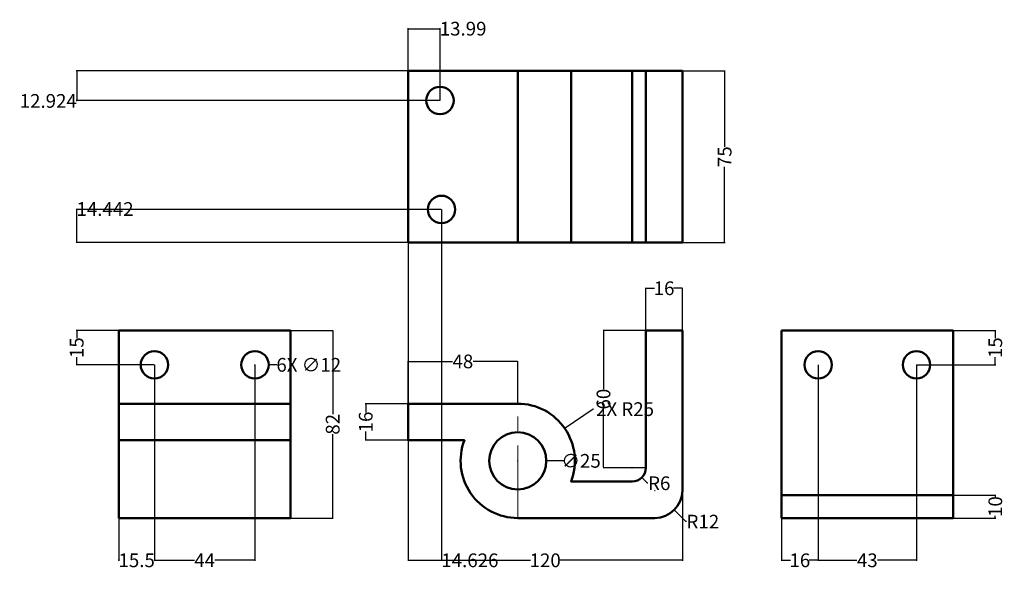
# Model space of a CAD drawing. Units: millimetres. Extents: x -15 to 416, y 9 to 249.
import ezdxf

# ---------------------------------------------------------------- set-up
doc = ezdxf.new("R2010")
doc.units = ezdxf.units.MM
doc.header["$MEASUREMENT"] = 0
doc.linetypes.add('CENTER', pattern=[50.8, 31.75, -6.35, 6.35, -6.35])
for name, color, linetype, lineweight in [('M-CNTR', 1, 'CENTER', 18), ('M-DIMS', 2, 'Continuous', 18), ('M-OUTL', 7, 'Continuous', 50)]:
    doc.layers.add(name, color=color, linetype=linetype, lineweight=lineweight)
doc.styles.get("Standard").update_dxf_attribs({"font": 'arial.ttf'})
doc.dimstyles.get("Standard").update_dxf_attribs({"dimtxt": 6, "dimasz": 0.18, "dimexe": 0.18, "dimexo": 0.0625, "dimgap": 0.09, "dimtad": 0, "dimtoh": 1, "dimdec": 0, "dimzin": 0, "dimdsep": 46, "dimtxsty": 'Standard', "dimcen": 0.09, "dimadec": 0, "dimazin": 0, "dimtfac": 1, "dimtdec": 0, "dimtofl": 0, "dimtmove": 0, "dimatfit": 3, "dimfxl": 1, "dimtolj": 1, "dimtzin": 0, "dimarcsym": 0})

# ---------------------------------------------------------------- blocks, each defined once
blk = doc.blocks.new('MTG-HOLE-D12')
blk.add_circle((6, 6), 6)
blk = doc.blocks.new('*D2')
at = {"layer": 'Defpoints', "color": 0, "transparency": 16777216}
for p in [(154.95, 65.07), (274.95, 43.07), (274.95, 12.57)]:
    blk.add_point(p, dxfattribs=at)
at = {"layer": 'M-DIMS', "color": 0, "lineweight": -2, "transparency": 16777216}
for p, q in [((154.95, 65.01), (154.95, 12.39)), ((274.95, 43.01), (274.95, 12.39)), ((155.13, 12.57), (208.52, 12.57)), ((274.77, 12.57), (221.37, 12.57))]:
    blk.add_line(p, q, dxfattribs=at)
at = {"layer": 'M-DIMS', "color": 0, "transparency": 16777216}
for points in [[(155.13, 12.6), (155.13, 12.54), (154.95, 12.57)], [(274.77, 12.6), (274.77, 12.54), (274.95, 12.57)]]:
    blk.add_solid(points, dxfattribs=at)
at = {"layer": 'M-DIMS', "color": 0, "transparency": 16777216, "insert": (214.95, 12.57), "char_height": 6, "attachment_point": 5}
blk.add_mtext('\\A1;120', dxfattribs=at)
blk = doc.blocks.new('*D3')
at = {"layer": 'Defpoints', "color": 0, "transparency": 16777216}
for p in [(103.5, 113.07), (103.5, 31.07), (122, 31.07)]:
    blk.add_point(p, dxfattribs=at)
at = {"layer": 'M-DIMS', "color": 0, "lineweight": -2, "transparency": 16777216}
for p, q in [((103.56, 113.07), (122.18, 113.07)), ((122, 112.89), (122, 76.43)), ((122, 31.25), (122, 67.71)), ((103.56, 31.07), (122.18, 31.07))]:
    blk.add_line(p, q, dxfattribs=at)
at = {"layer": 'M-DIMS', "color": 0, "transparency": 16777216}
for points in [[(121.97, 112.89), (122.03, 112.89), (122, 113.07)], [(121.97, 31.25), (122.03, 31.25), (122, 31.07)]]:
    blk.add_solid(points, dxfattribs=at)
at = {"layer": 'M-DIMS', "color": 0, "transparency": 16777216, "insert": (122, 72.07), "char_height": 6, "attachment_point": 5, "rotation": 90}
blk.add_mtext('\\A1;82', dxfattribs=at)
blk = doc.blocks.new('*D4')
at = {"layer": 'Defpoints', "color": 0, "transparency": 16777216}
for p in [(274.95, 226.61), (274.95, 151.61), (293.45, 151.61)]:
    blk.add_point(p, dxfattribs=at)
at = {"layer": 'M-DIMS', "color": 0, "lineweight": -2, "transparency": 16777216}
for p, q in [((275.01, 226.61), (293.63, 226.61)), ((293.45, 226.43), (293.45, 193.49)), ((293.45, 151.79), (293.45, 184.72)), ((275.01, 151.61), (293.63, 151.61))]:
    blk.add_line(p, q, dxfattribs=at)
at = {"layer": 'M-DIMS', "color": 0, "transparency": 16777216}
for points in [[(293.42, 226.43), (293.48, 226.43), (293.45, 226.61)], [(293.42, 151.79), (293.48, 151.79), (293.45, 151.61)]]:
    blk.add_solid(points, dxfattribs=at)
at = {"layer": 'M-DIMS', "color": 0, "transparency": 16777216, "insert": (293.45, 189.11), "char_height": 6, "attachment_point": 5, "rotation": 90}
blk.add_mtext('\\A1;75', dxfattribs=at)
blk = doc.blocks.new('*D5')
at = {"layer": 'Defpoints', "color": 0, "transparency": 16777216}
for p in [(202.95, 99.57), (154.95, 81.07), (202.95, 81.07)]:
    blk.add_point(p, dxfattribs=at)
at = {"layer": 'M-DIMS', "color": 0, "lineweight": -2, "transparency": 16777216}
for p, q in [((154.95, 81.13), (154.95, 99.75)), ((155.13, 99.57), (174.43, 99.57)), ((202.77, 99.57), (183.46, 99.57)), ((202.95, 81.13), (202.95, 99.75))]:
    blk.add_line(p, q, dxfattribs=at)
at = {"layer": 'M-DIMS', "color": 0, "transparency": 16777216}
for points in [[(155.13, 99.6), (155.13, 99.54), (154.95, 99.57)], [(202.77, 99.6), (202.77, 99.54), (202.95, 99.57)]]:
    blk.add_solid(points, dxfattribs=at)
at = {"layer": 'M-DIMS', "color": 0, "transparency": 16777216, "insert": (178.95, 99.57), "char_height": 6, "attachment_point": 5}
blk.add_mtext('\\A1;48', dxfattribs=at)
blk = doc.blocks.new('*D6')
at = {"layer": 'Defpoints', "color": 0, "transparency": 16777216}
for p in [(136.45, 81.07), (154.95, 81.07), (154.95, 65.07)]:
    blk.add_point(p, dxfattribs=at)
at = {"layer": 'M-DIMS', "color": 0, "lineweight": -2, "transparency": 16777216}
for p, q in [((154.88, 81.07), (136.27, 81.07)), ((136.45, 80.89), (136.45, 77.17)), ((136.45, 65.25), (136.45, 68.97)), ((154.88, 65.07), (136.27, 65.07))]:
    blk.add_line(p, q, dxfattribs=at)
at = {"layer": 'M-DIMS', "color": 0, "transparency": 16777216}
for points in [[(136.42, 80.89), (136.48, 80.89), (136.45, 81.07)], [(136.42, 65.25), (136.48, 65.25), (136.45, 65.07)]]:
    blk.add_solid(points, dxfattribs=at)
at = {"layer": 'M-DIMS', "color": 0, "transparency": 16777216, "insert": (136.45, 73.07), "char_height": 6, "attachment_point": 5, "rotation": 90}
blk.add_mtext('\\A1;16', dxfattribs=at)
blk = doc.blocks.new('*D7')
at = {"layer": 'Defpoints', "color": 0, "transparency": 16777216}
for p in [(274.95, 131.57), (258.95, 113.07), (274.95, 113.07)]:
    blk.add_point(p, dxfattribs=at)
at = {"layer": 'M-DIMS', "color": 0, "lineweight": -2, "transparency": 16777216}
for p, q in [((258.95, 113.13), (258.95, 131.75)), ((259.13, 131.57), (262.84, 131.57)), ((274.77, 131.57), (271.05, 131.57)), ((274.95, 113.13), (274.95, 131.75))]:
    blk.add_line(p, q, dxfattribs=at)
at = {"layer": 'M-DIMS', "color": 0, "transparency": 16777216}
for points in [[(259.13, 131.6), (259.13, 131.54), (258.95, 131.57)], [(274.77, 131.6), (274.77, 131.54), (274.95, 131.57)]]:
    blk.add_solid(points, dxfattribs=at)
at = {"layer": 'M-DIMS', "color": 0, "transparency": 16777216, "insert": (266.95, 131.57), "char_height": 6, "attachment_point": 5}
blk.add_mtext('\\A1;16', dxfattribs=at)
blk = doc.blocks.new('*D8')
at = {"layer": 'Defpoints', "color": 0, "transparency": 16777216}
for p in [(240.45, 113.07), (258.95, 113.07), (258.95, 53.07)]:
    blk.add_point(p, dxfattribs=at)
at = {"layer": 'M-DIMS', "color": 0, "lineweight": -2, "transparency": 16777216}
for p, q in [((258.88, 113.07), (240.27, 113.07)), ((240.45, 112.89), (240.45, 87.46)), ((240.45, 53.25), (240.45, 78.68)), ((258.88, 53.07), (240.27, 53.07))]:
    blk.add_line(p, q, dxfattribs=at)
at = {"layer": 'M-DIMS', "color": 0, "transparency": 16777216}
for points in [[(240.42, 112.89), (240.48, 112.89), (240.45, 113.07)], [(240.42, 53.25), (240.48, 53.25), (240.45, 53.07)]]:
    blk.add_solid(points, dxfattribs=at)
at = {"layer": 'M-DIMS', "color": 0, "transparency": 16777216, "insert": (240.45, 83.07), "char_height": 6, "attachment_point": 5, "rotation": 90}
blk.add_mtext('\\A1;60', dxfattribs=at)
blk = doc.blocks.new('*D9')
at = {"layer": 'Defpoints', "color": 0, "transparency": 16777216}
for p in [(43.999556, 98.070817), (28.499556, 31.070817), (43.999556, 12.570817)]:
    blk.add_point(p, dxfattribs=at)
at = {"layer": 'M-DIMS', "color": 0, "lineweight": -2, "transparency": 16777216}
for p, q in [((43.999556, 98.008317), (43.999556, 12.390817)), ((28.499556, 31.008317), (28.499556, 12.390817)), ((28.319556, 12.570817), (28.139556, 12.570817)), ((44.179556, 12.570817), (44.359556, 12.570817))]:
    blk.add_line(p, q, dxfattribs=at)
at = {"layer": 'M-DIMS', "color": 0, "transparency": 16777216}
for points in [[(28.319556, 12.600817), (28.319556, 12.540817), (28.499556, 12.570817)], [(44.179556, 12.600817), (44.179556, 12.540817), (43.999556, 12.570817)]]:
    blk.add_solid(points, dxfattribs=at)
at = {"layer": 'M-DIMS', "color": 0, "transparency": 16777216, "insert": (36.249556, 12.570817), "char_height": 6, "attachment_point": 5}
blk.add_mtext('\\A1;15.5', dxfattribs=at)
blk = doc.blocks.new('*D10')
at = {"layer": 'Defpoints', "color": 0, "transparency": 16777216}
for p in [(44, 98.07), (88, 98.07), (88, 12.57)]:
    blk.add_point(p, dxfattribs=at)
at = {"layer": 'M-DIMS', "color": 0, "lineweight": -2, "transparency": 16777216}
for p, q in [((44, 98.01), (44, 12.39)), ((88, 98.01), (88, 12.39)), ((44.18, 12.57), (61.5, 12.57)), ((87.82, 12.57), (70.5, 12.57))]:
    blk.add_line(p, q, dxfattribs=at)
at = {"layer": 'M-DIMS', "color": 0, "transparency": 16777216}
for points in [[(44.18, 12.6), (44.18, 12.54), (44, 12.57)], [(87.82, 12.6), (87.82, 12.54), (88, 12.57)]]:
    blk.add_solid(points, dxfattribs=at)
at = {"layer": 'M-DIMS', "color": 0, "transparency": 16777216, "insert": (66, 12.57), "char_height": 6, "attachment_point": 5}
blk.add_mtext('\\A1;44', dxfattribs=at)
blk = doc.blocks.new('*D11')
at = {"layer": 'Defpoints', "color": 0, "transparency": 16777216}
for p in [(28.5, 113.07), (10, 98.07), (44, 98.07)]:
    blk.add_point(p, dxfattribs=at)
at = {"layer": 'M-DIMS', "color": 0, "lineweight": -2, "transparency": 16777216}
for p, q in [((28.44, 113.07), (9.82, 113.07)), ((10, 112.89), (10, 109.7)), ((10, 98.25), (10, 101.44)), ((43.94, 98.07), (9.82, 98.07))]:
    blk.add_line(p, q, dxfattribs=at)
at = {"layer": 'M-DIMS', "color": 0, "transparency": 16777216}
for points in [[(9.97, 112.89), (10.03, 112.89), (10, 113.07)], [(9.97, 98.25), (10.03, 98.25), (10, 98.07)]]:
    blk.add_solid(points, dxfattribs=at)
at = {"layer": 'M-DIMS', "color": 0, "transparency": 16777216, "insert": (10, 105.57), "char_height": 6, "attachment_point": 5, "rotation": 90}
blk.add_mtext('\\A1;15', dxfattribs=at)
blk = doc.blocks.new('*D12')
at = {"layer": 'Defpoints', "color": 0, "transparency": 16777216}
for p in [(334.35, 98.07), (318.35, 31.07), (334.35, 12.57)]:
    blk.add_point(p, dxfattribs=at)
at = {"layer": 'M-DIMS', "color": 0, "lineweight": -2, "transparency": 16777216}
for p, q in [((334.35, 98.01), (334.35, 12.39)), ((318.35, 31.01), (318.35, 12.39)), ((318.53, 12.57), (322.25, 12.57)), ((334.17, 12.57), (330.45, 12.57))]:
    blk.add_line(p, q, dxfattribs=at)
at = {"layer": 'M-DIMS', "color": 0, "transparency": 16777216}
for points in [[(318.53, 12.6), (318.53, 12.54), (318.35, 12.57)], [(334.17, 12.6), (334.17, 12.54), (334.35, 12.57)]]:
    blk.add_solid(points, dxfattribs=at)
at = {"layer": 'M-DIMS', "color": 0, "transparency": 16777216, "insert": (326.35, 12.57), "char_height": 6, "attachment_point": 5}
blk.add_mtext('\\A1;16', dxfattribs=at)
blk = doc.blocks.new('*D13')
at = {"layer": 'Defpoints', "color": 0, "transparency": 16777216}
for p in [(334.35, 98.07), (377.35, 98.07), (377.35, 12.57)]:
    blk.add_point(p, dxfattribs=at)
at = {"layer": 'M-DIMS', "color": 0, "lineweight": -2, "transparency": 16777216}
for p, q in [((334.35, 98.01), (334.35, 12.39)), ((377.35, 98.01), (377.35, 12.39)), ((334.53, 12.57), (351.34, 12.57)), ((377.17, 12.57), (360.36, 12.57))]:
    blk.add_line(p, q, dxfattribs=at)
at = {"layer": 'M-DIMS', "color": 0, "transparency": 16777216}
for points in [[(334.53, 12.6), (334.53, 12.54), (334.35, 12.57)], [(377.17, 12.6), (377.17, 12.54), (377.35, 12.57)]]:
    blk.add_solid(points, dxfattribs=at)
at = {"layer": 'M-DIMS', "color": 0, "transparency": 16777216, "insert": (355.85, 12.57), "char_height": 6, "attachment_point": 5}
blk.add_mtext('\\A1;43', dxfattribs=at)
blk = doc.blocks.new('*D14')
at = {"layer": 'Defpoints', "color": 0, "transparency": 16777216}
for p in [(393.35, 113.07), (411.85, 113.07), (377.35, 98.07)]:
    blk.add_point(p, dxfattribs=at)
at = {"layer": 'M-DIMS', "color": 0, "lineweight": -2, "transparency": 16777216}
for p, q in [((393.41, 113.07), (412.03, 113.07)), ((411.85, 112.89), (411.85, 109.7)), ((411.85, 98.25), (411.85, 101.44)), ((377.41, 98.07), (412.03, 98.07))]:
    blk.add_line(p, q, dxfattribs=at)
at = {"layer": 'M-DIMS', "color": 0, "transparency": 16777216}
for points in [[(411.82, 112.89), (411.88, 112.89), (411.85, 113.07)], [(411.82, 98.25), (411.88, 98.25), (411.85, 98.07)]]:
    blk.add_solid(points, dxfattribs=at)
at = {"layer": 'M-DIMS', "color": 0, "transparency": 16777216, "insert": (411.85, 105.57), "char_height": 6, "attachment_point": 5, "rotation": 90}
blk.add_mtext('\\A1;15', dxfattribs=at)
blk = doc.blocks.new('*D15')
at = {"layer": 'Defpoints', "color": 0, "transparency": 16777216}
for p in [(168.94, 245.11), (154.95, 226.61), (168.94, 213.68)]:
    blk.add_point(p, dxfattribs=at)
at = {"layer": 'M-DIMS', "color": 0, "lineweight": -2, "transparency": 16777216}
for p, q in [((154.95, 226.67), (154.95, 245.29)), ((155.13, 245.11), (168.76, 245.11)), ((168.94, 213.75), (168.94, 245.29)), ((168.94, 245.11), (169.12, 245.11))]:
    blk.add_line(p, q, dxfattribs=at)
at = {"layer": 'M-DIMS', "color": 0, "transparency": 16777216}
for points in [[(155.13, 245.14), (155.13, 245.08), (154.95, 245.11)], [(168.76, 245.14), (168.76, 245.08), (168.94, 245.11)]]:
    blk.add_solid(points, dxfattribs=at)
at = {"layer": 'M-DIMS', "color": 0, "transparency": 16777216, "insert": (179.05, 245.11), "char_height": 6, "attachment_point": 5}
blk.add_mtext('\\A1;13.99', dxfattribs=at)
blk = doc.blocks.new('*D16')
at = {"layer": 'Defpoints', "color": 0, "transparency": 16777216}
for p in [(154.95, 226.61), (10, 213.68), (168.94, 213.68)]:
    blk.add_point(p, dxfattribs=at)
at = {"layer": 'M-DIMS', "color": 0, "lineweight": -2, "transparency": 16777216}
for p, q in [((154.88, 226.61), (9.82, 226.61)), ((10, 226.43), (10, 213.86)), ((168.87, 213.68), (9.82, 213.68)), ((10, 213.5), (9.82, 213.5)), ((10, 213.68), (10, 213.5))]:
    blk.add_line(p, q, dxfattribs=at)
at = {"layer": 'M-DIMS', "color": 0, "transparency": 16777216}
for points in [[(9.97, 226.43), (10.03, 226.43), (10, 226.61)], [(9.97, 213.86), (10.03, 213.86), (10, 213.68)]]:
    blk.add_solid(points, dxfattribs=at)
at = {"layer": 'M-DIMS', "color": 0, "transparency": 16777216, "insert": (-2.43, 213.5), "char_height": 6, "attachment_point": 5}
blk.add_mtext('\\A1;12.924', dxfattribs=at)
blk = doc.blocks.new('*D17')
at = {"layer": 'Defpoints', "color": 0, "transparency": 16777216}
for p in [(169.57, 166.05), (154.95, 151.61), (169.57, 12.57)]:
    blk.add_point(p, dxfattribs=at)
at = {"layer": 'M-DIMS', "color": 0, "lineweight": -2, "transparency": 16777216}
for p, q in [((169.57, 165.99), (169.57, 12.39)), ((154.95, 151.55), (154.95, 12.39)), ((155.13, 12.57), (169.39, 12.57)), ((169.57, 12.57), (169.75, 12.57))]:
    blk.add_line(p, q, dxfattribs=at)
at = {"layer": 'M-DIMS', "color": 0, "transparency": 16777216}
for points in [[(155.13, 12.6), (155.13, 12.54), (154.95, 12.57)], [(169.39, 12.6), (169.39, 12.54), (169.57, 12.57)]]:
    blk.add_solid(points, dxfattribs=at)
at = {"layer": 'M-DIMS', "color": 0, "transparency": 16777216, "insert": (182.01, 12.57), "char_height": 6, "attachment_point": 5}
blk.add_mtext('\\A1;14.626', dxfattribs=at)
blk = doc.blocks.new('*D18')
at = {"layer": 'Defpoints', "color": 0, "transparency": 16777216}
for p in [(10, 166.05), (169.57, 166.05), (154.95, 151.61)]:
    blk.add_point(p, dxfattribs=at)
at = {"layer": 'M-DIMS', "color": 0, "lineweight": -2, "transparency": 16777216}
for p, q in [((169.51, 166.05), (9.82, 166.05)), ((10, 166.05), (10, 166.23)), ((10, 166.23), (10.18, 166.23)), ((10, 151.79), (10, 165.87)), ((154.88, 151.61), (9.82, 151.61))]:
    blk.add_line(p, q, dxfattribs=at)
at = {"layer": 'M-DIMS', "color": 0, "transparency": 16777216}
for points in [[(9.97, 165.87), (10.03, 165.87), (10, 166.05)], [(9.97, 151.79), (10.03, 151.79), (10, 151.61)]]:
    blk.add_solid(points, dxfattribs=at)
at = {"layer": 'M-DIMS', "color": 0, "transparency": 16777216, "insert": (22.41, 166.23), "char_height": 6, "attachment_point": 5}
blk.add_mtext('\\A1;14.442', dxfattribs=at)
blk = doc.blocks.new('*D19')
at = {"layer": 'Defpoints', "color": 0, "transparency": 16777216}
for p in [(393.35, 41.07), (393.35, 31.07), (411.85, 31.07)]:
    blk.add_point(p, dxfattribs=at)
at = {"layer": 'M-DIMS', "color": 0, "lineweight": -2, "transparency": 16777216}
for p, q in [((393.41, 41.07), (412.03, 41.07)), ((411.85, 40.89), (411.85, 40.17)), ((393.41, 31.07), (412.03, 31.07)), ((411.85, 31.25), (411.85, 31.98))]:
    blk.add_line(p, q, dxfattribs=at)
at = {"layer": 'M-DIMS', "color": 0, "transparency": 16777216}
for points in [[(411.82, 40.89), (411.88, 40.89), (411.85, 41.07)], [(411.82, 31.25), (411.88, 31.25), (411.85, 31.07)]]:
    blk.add_solid(points, dxfattribs=at)
at = {"layer": 'M-DIMS', "color": 0, "transparency": 16777216, "insert": (411.85, 36.07), "char_height": 6, "attachment_point": 5, "rotation": 90}
blk.add_mtext('\\A1;10', dxfattribs=at)
blk = doc.blocks.new('*D20')
at = {"layer": 'Defpoints', "color": 0, "transparency": 16777216}
for p in [(190.45, 56.07), (215.45, 56.07)]:
    blk.add_point(p, dxfattribs=at)
at = {"layer": 'M-DIMS', "color": 0, "lineweight": -2, "transparency": 16777216}
for p, q in [((202.86, 56.07), (203.04, 56.07)), ((202.95, 55.98), (202.95, 56.16)), ((222.95, 56.07), (215.63, 56.07))]:
    blk.add_line(p, q, dxfattribs=at)
at = {"layer": 'M-DIMS', "color": 0, "transparency": 16777216}
blk.add_solid([(215.63, 56.1), (215.63, 56.04), (215.45, 56.07)], dxfattribs=at)
at = {"layer": 'M-DIMS', "color": 0, "transparency": 16777216, "insert": (230.62, 56.07), "char_height": 6, "attachment_point": 5}
blk.add_mtext('\\A1;∅25', dxfattribs=at)
blk = doc.blocks.new('*D21')
at = {"layer": 'Defpoints', "color": 0, "transparency": 16777216}
for p in [(223.56, 70.21), (202.95, 56.07)]:
    blk.add_point(p, dxfattribs=at)
at = {"layer": 'M-DIMS', "color": 0, "lineweight": -2, "transparency": 16777216}
for p, q in [((235.93, 78.7), (223.71, 70.31)), ((236.11, 78.7), (235.93, 78.7)), ((202.86, 56.07), (203.04, 56.07)), ((202.95, 55.98), (202.95, 56.16))]:
    blk.add_line(p, q, dxfattribs=at)
at = {"layer": 'M-DIMS', "color": 0, "transparency": 16777216}
blk.add_solid([(223.69, 70.34), (223.73, 70.29), (223.56, 70.21)], dxfattribs=at)
at = {"layer": 'M-DIMS', "color": 0, "transparency": 16777216, "insert": (249.89, 78.7), "char_height": 6, "attachment_point": 5}
blk.add_mtext('\\A1;2X R25', dxfattribs=at)
blk = doc.blocks.new('*D22')
at = {"layer": 'Defpoints', "color": 0, "transparency": 16777216}
for p in [(262.95, 43.07), (271.43, 34.59)]:
    blk.add_point(p, dxfattribs=at)
at = {"layer": 'M-DIMS', "color": 0, "lineweight": -2, "transparency": 16777216}
for p, q in [((262.95, 42.98), (262.95, 43.16)), ((262.86, 43.07), (263.04, 43.07)), ((276.52, 29.49), (271.56, 34.46)), ((276.7, 29.49), (276.52, 29.49))]:
    blk.add_line(p, q, dxfattribs=at)
at = {"layer": 'M-DIMS', "color": 0, "transparency": 16777216}
blk.add_solid([(271.58, 34.48), (271.54, 34.44), (271.43, 34.59)], dxfattribs=at)
at = {"layer": 'M-DIMS', "color": 0, "transparency": 16777216, "insert": (283.93, 29.49), "char_height": 6, "attachment_point": 5}
blk.add_mtext('\\A1;R12', dxfattribs=at)
blk = doc.blocks.new('*D23')
at = {"layer": 'Defpoints', "color": 0, "transparency": 16777216}
for p in [(252.95, 53.07), (257.19, 48.83)]:
    blk.add_point(p, dxfattribs=at)
at = {"layer": 'M-DIMS', "color": 0, "lineweight": -2, "transparency": 16777216}
for p, q in [((252.86, 53.07), (253.04, 53.07)), ((252.95, 52.98), (252.95, 53.16)), ((259.73, 46.28), (257.32, 48.7)), ((259.91, 46.28), (259.73, 46.28))]:
    blk.add_line(p, q, dxfattribs=at)
at = {"layer": 'M-DIMS', "color": 0, "transparency": 16777216}
blk.add_solid([(257.34, 48.72), (257.29, 48.68), (257.19, 48.83)], dxfattribs=at)
at = {"layer": 'M-DIMS', "color": 0, "transparency": 16777216, "insert": (264.84, 46.28), "char_height": 6, "attachment_point": 5}
blk.add_mtext('\\A1;R6', dxfattribs=at)
blk = doc.blocks.new('*D24')
at = {"layer": 'Defpoints', "color": 0, "transparency": 16777216}
for p in [(82, 98.07), (94, 98.07)]:
    blk.add_point(p, dxfattribs=at)
at = {"layer": 'M-DIMS', "color": 0, "lineweight": -2, "transparency": 16777216}
for p, q in [((87.91, 98.07), (88.09, 98.07)), ((88, 97.98), (88, 98.16)), ((97.6, 98.07), (94.18, 98.07))]:
    blk.add_line(p, q, dxfattribs=at)
at = {"layer": 'M-DIMS', "color": 0, "transparency": 16777216}
blk.add_solid([(94.18, 98.1), (94.18, 98.04), (94, 98.07)], dxfattribs=at)
at = {"layer": 'M-DIMS', "color": 0, "transparency": 16777216, "insert": (111.52, 98.07), "char_height": 6, "attachment_point": 5}
blk.add_mtext('\\A1;6X ∅12', dxfattribs=at)

msp = doc.modelspace()

# ---------------------------------------------------------------- linework, layer by layer
at = {"layer": 'M-CNTR'}
msp.add_line((202.9462, 31.0708), (202.9462, 81.0708), dxfattribs=at)
at = {"layer": 'M-OUTL'}
for p, q in [((202.9462, 151.6075), (202.9462, 226.6075)), ((226.27, 151.6075), (226.27, 226.6075)), ((252.9462, 151.6075), (252.9462, 226.6075)), ((258.9462, 226.6075), (258.9462, 151.6075)), ((28.4996, 81.0708), (103.4996, 81.0708)), ((28.4996, 65.0708), (103.4996, 65.0708)), ((318.3518, 41.0708), (393.3518, 41.0708))]:
    msp.add_line(p, q, dxfattribs=at)
for points in [[(274.9462, 151.6075), (274.9462, 226.6075), (154.9462, 226.6075), (154.9462, 151.6075)], [(28.4996, 113.0708), (103.4996, 113.0708), (103.4996, 31.0708), (28.4996, 31.0708)], [(318.3518, 113.0708), (318.3518, 31.0708), (393.3518, 31.0708), (393.3518, 113.0708), (390.3518, 113.0708)]]:
    msp.add_lwpolyline(points, close=True, dxfattribs=at)
msp.add_lwpolyline([(258.9462, 113.0708), (274.9462, 113.0708), (274.9462, 43.0708, -0.41421356), (262.9462, 31.0708), (202.9462, 31.0708, -0.52668378), (179.6224, 65.0708), (154.9462, 65.0708), (154.9462, 81.0708), (202.9462, 81.0708, -0.52668378), (226.27, 47.0708), (252.9462, 47.0708, 0.41421356), (258.9462, 53.0708)], format="xyb", close=True, dxfattribs=at)
msp.add_circle((202.9462, 56.0708), 12.5, dxfattribs=at)

# ---------------------------------------------------------------- block references
for p in [(162.9368, 207.6839), (163.5728, 160.0493), (38, 92.071), (82, 92.071), (328.3523, 92.071), (371.3523, 92.071)]:
    msp.add_blockref('MTG-HOLE-D12', p, dxfattribs=at)

# ---------------------------------------------------------------- dimensions: what is measured, and where the dimension line sits
at = {"layer": 'M-DIMS'}
for base, p1, p2, override, picture, middle in [((168.9364, 245.1075), (154.9462, 226.6075), (168.9364, 213.6837), {"dimdec": 2, "dimlfac": 1, "dimrnd": 0, "dimzin": 0, "dimdsep": 46, "dimlunit": 2}, '*D15', (179.0536, 245.1075)), ((169.5724, 12.5708), (154.9462, 151.6075), (169.5724, 166.0491), {"dimdec": 3, "dimlfac": 1, "dimrnd": 0, "dimzin": 0, "dimdsep": 46, "dimlunit": 2}, '*D17', (182.0122, 12.5708)), ((274.9462, 131.5708), (258.9462, 113.0708), (274.9462, 113.0708), {"dimdec": 0, "dimlfac": 1, "dimrnd": 0, "dimzin": 0, "dimdsep": 46, "dimlunit": 2}, '*D7', (266.9462, 131.5708)), ((202.9462, 99.5708), (154.9462, 81.0708), (202.9462, 81.0708), {"dimdec": 0, "dimlfac": 1, "dimrnd": 0, "dimzin": 0, "dimdsep": 46, "dimlunit": 2}, '*D5', (178.9462, 99.5708)), ((43.9996, 12.5708), (28.4996, 31.0708), (43.9996, 98.0708), {"dimdec": 1, "dimlfac": 1, "dimrnd": 0, "dimzin": 0, "dimdsep": 46, "dimlunit": 2}, '*D9', (36.2496, 12.5708)), ((87.9996, 12.5708), (43.9996, 98.0708), (87.9996, 98.0708), {"dimdec": 0, "dimlfac": 1, "dimrnd": 0, "dimzin": 0, "dimdsep": 46, "dimlunit": 2}, '*D10', (65.9996, 12.5708)), ((334.3518, 12.5708), (318.3518, 31.0708), (334.3518, 98.0708), {"dimdec": 0, "dimlfac": 1, "dimrnd": 0, "dimzin": 0, "dimdsep": 46, "dimlunit": 2}, '*D12', (326.3518, 12.5708)), ((377.3518, 12.5708), (334.3518, 98.0708), (377.3518, 98.0708), {"dimdec": 0, "dimlfac": 1, "dimrnd": 0, "dimzin": 0, "dimdsep": 46, "dimlunit": 2}, '*D13', (355.8518, 12.5708)), ((274.9462, 12.5708), (154.9462, 65.0708), (274.9462, 43.0708), {"dimdec": 0, "dimlfac": 1, "dimrnd": 0, "dimzin": 0, "dimdsep": 46, "dimlunit": 2}, '*D2', (214.9462, 12.5708))]:
    dim = msp.add_linear_dim(base=base, p1=p1, p2=p2, dimstyle='Standard', override=override, dxfattribs=at)
    dim.commit()
    dim.dimension.update_dxf_attribs({"geometry": picture, "text_midpoint": middle})
for base, p1, p2, angle, override, picture, middle in [((9.9996, 213.6837), (154.9462, 226.6075), (168.9364, 213.6837), 90, {"dimdec": 3, "dimlfac": 1, "dimrnd": 0, "dimzin": 0, "dimdsep": 46, "dimlunit": 2}, '*D16', (-2.4301, 213.5037)), ((293.4462, 151.6075), (274.9462, 226.6075), (274.9462, 151.6075), 270, {"dimdec": 0, "dimlfac": 1, "dimrnd": 0, "dimzin": 0, "dimdsep": 46, "dimlunit": 2}, '*D4', (293.4462, 189.1075)), ((9.9996, 166.0491), (154.9462, 151.6075), (169.5724, 166.0491), 90, {"dimdec": 3, "dimlfac": 1, "dimrnd": 0, "dimzin": 0, "dimdsep": 46, "dimlunit": 2}, '*D18', (22.4108, 166.2291)), ((9.9996, 98.0708), (28.4996, 113.0708), (43.9996, 98.0708), 90, {"dimdec": 0, "dimlfac": 1, "dimrnd": 0, "dimzin": 0, "dimdsep": 46, "dimlunit": 2}, '*D11', (9.9996, 105.5708)), ((121.9996, 31.0708), (103.4996, 113.0708), (103.4996, 31.0708), 270, {"dimdec": 0, "dimlfac": 1, "dimrnd": 0, "dimzin": 0, "dimdsep": 46, "dimlunit": 2}, '*D3', (121.9996, 72.0708)), ((240.4462, 113.0708), (258.9462, 53.0708), (258.9462, 113.0708), 90, {"dimdec": 0, "dimlfac": 1, "dimrnd": 0, "dimzin": 0, "dimdsep": 46, "dimlunit": 2}, '*D8', (240.4462, 83.0708)), ((411.8518, 113.0708), (377.3518, 98.0708), (393.3518, 113.0708), 90, {"dimdec": 0, "dimlfac": 1, "dimrnd": 0, "dimzin": 0, "dimdsep": 46, "dimlunit": 2}, '*D14', (411.8518, 105.5708)), ((136.4462, 81.0708), (154.9462, 65.0708), (154.9462, 81.0708), 90, {"dimdec": 0, "dimlfac": 1, "dimrnd": 0, "dimzin": 0, "dimdsep": 46, "dimlunit": 2}, '*D6', (136.4462, 73.0708)), ((411.8518, 31.0708), (393.3518, 41.0708), (393.3518, 31.0708), 90, {"dimdec": 0, "dimlfac": 1, "dimrnd": 0, "dimzin": 0, "dimdsep": 46, "dimlunit": 2}, '*D19', (411.8518, 36.0708))]:
    dim = msp.add_linear_dim(base=base, p1=p1, p2=p2, angle=angle, dimstyle='Standard', override=override, dxfattribs=at)
    dim.commit()
    dim.dimension.update_dxf_attribs({"geometry": picture, "text_midpoint": middle})
dim = msp.add_diameter_dim_2p(p1=(81.9996, 98.0706), p2=(93.9996, 98.071), text='6X <>', dimstyle='Standard', override={"dimdec": 0, "dimlfac": 1, "dimrnd": 0, "dimzin": 0, "dimdsep": 46, "dimlunit": 2}, dxfattribs=at)
dim.commit()
dim.dimension.update_dxf_attribs({"geometry": '*D24', "text_midpoint": (97.5996, 98.0711), "dimtype": 163})
dim = msp.add_radius_dim(center=(202.9462, 56.0708), mpoint=(223.5618, 70.2128), text='2X <>', dimstyle='Standard', override={"dimdec": 0, "dimlfac": 1, "dimrnd": 0, "dimzin": 0, "dimdsep": 46, "dimlunit": 2}, dxfattribs=at)
dim.commit()
dim.dimension.update_dxf_attribs({"geometry": '*D21', "text_midpoint": (249.8894, 78.6981), "dimtype": 164})
dim = msp.add_diameter_dim_2p(p1=(190.4462, 56.0706), p2=(215.4462, 56.071), dimstyle='Standard', override={"dimdec": 0, "dimlfac": 1, "dimrnd": 0, "dimzin": 0, "dimdsep": 46, "dimlunit": 2}, dxfattribs=at)
dim.commit()
dim.dimension.update_dxf_attribs({"geometry": '*D20', "text_midpoint": (222.9462, 56.0711), "dimtype": 163})
for center, mpoint, picture, middle in [((252.9462, 53.0708), (257.1888, 48.8282), '*D23', (264.84, 46.2826)), ((262.9462, 43.0708), (271.4315, 34.5855), '*D22', (283.9304, 29.4944))]:
    dim = msp.add_radius_dim(center=center, mpoint=mpoint, dimstyle='Standard', override={"dimdec": 0, "dimlfac": 1, "dimrnd": 0, "dimzin": 0, "dimdsep": 46, "dimlunit": 2}, dxfattribs=at)
    dim.commit()
    dim.dimension.update_dxf_attribs({"geometry": picture, "text_midpoint": middle, "dimtype": 164})

doc.saveas('drawing.dxf')
